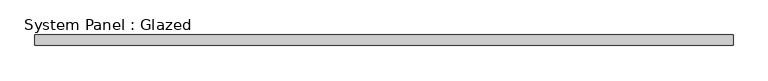
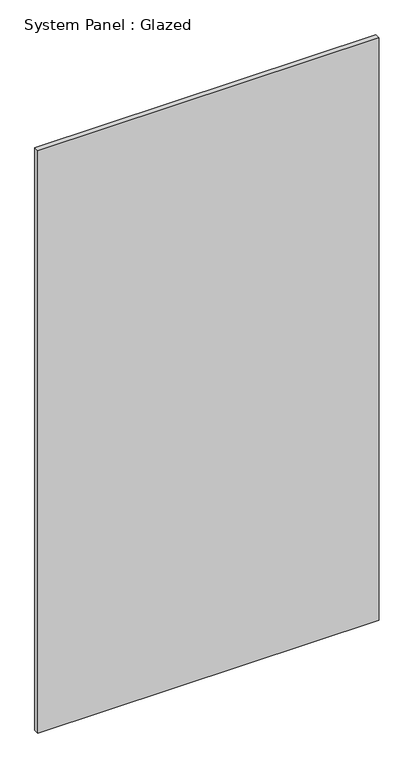
"""IFC4 building model written with IfcOpenShell, lengths in millimetres: plate geometry, System Panel : Glazed."""

from ifc_helpers import new_model, si_unit, origin, origin_with_axes, place, context, project, spatial, polyline, outline, extrude, source, transform, mapped, element, save


def system_panel_glazed_4e689a8f(model_context):
    return source(origin(), model_context, "Body", "SweptSolid", [
        extrude(outline(polyline([(831.5259936, 24.5), (-831.5259936, 24.5), (-831.5259936, 49.5), (831.5259936, 49.5), (831.5259936, 24.5)])), origin_with_axes(), (0.0, 0.0, 1.0), 3000.0),
    ])


if __name__ == "__main__":
    model = new_model("IFC4")
    model_context = context("Model", 3, world=origin())
    ifc_project = project(units=[si_unit("LENGTHUNIT", "METRE", prefix="MILLI")], contexts=[model_context])
    site = spatial("IfcSite", under=ifc_project)
    building = spatial("IfcBuilding", under=site)
    placement = place(None, origin())
    system_panel_glazed_shape = system_panel_glazed_4e689a8f(model_context)
    element("IfcPlate", 1, ObjectType="System Panel : Glazed", at=placement, inside=building, context=model_context, shape_type="MappedRepresentation", body=[
        mapped(system_panel_glazed_shape, transform((0.0, 0.0, 0.0), x_axis=(1.0, 0.0, 0.0), y_axis=(0.0, 1.0, 0.0), z_axis=(0.0, 0.0, 1.0))),
    ])
    save(model, "model.ifc")

# Revit data of these elements
# Type "System Panel : Glazed"
#   Keynote = "H11"
#   Construction Type Id = "GSP4R"
#   Analytic Construction = "1/8 in Pilkington single glazing"
#   Visual Light Transmittance = 0.9
#   Solar Heat Gain Coefficient = 0.86
#   Heat Transfer Coefficient (U) = 6.7069 W/(m²·K)
#   Define Thermal Properties by = 1
# Element 1 (IfcPlate, "System Panel : Glazed")
#   Materials on its faces: "Glass"
# Materials
#   "Glass": class "Glass", colour RGB 0 128 192, transparency 0.9, Description = "Soda Lime Glass", Cost = 0
